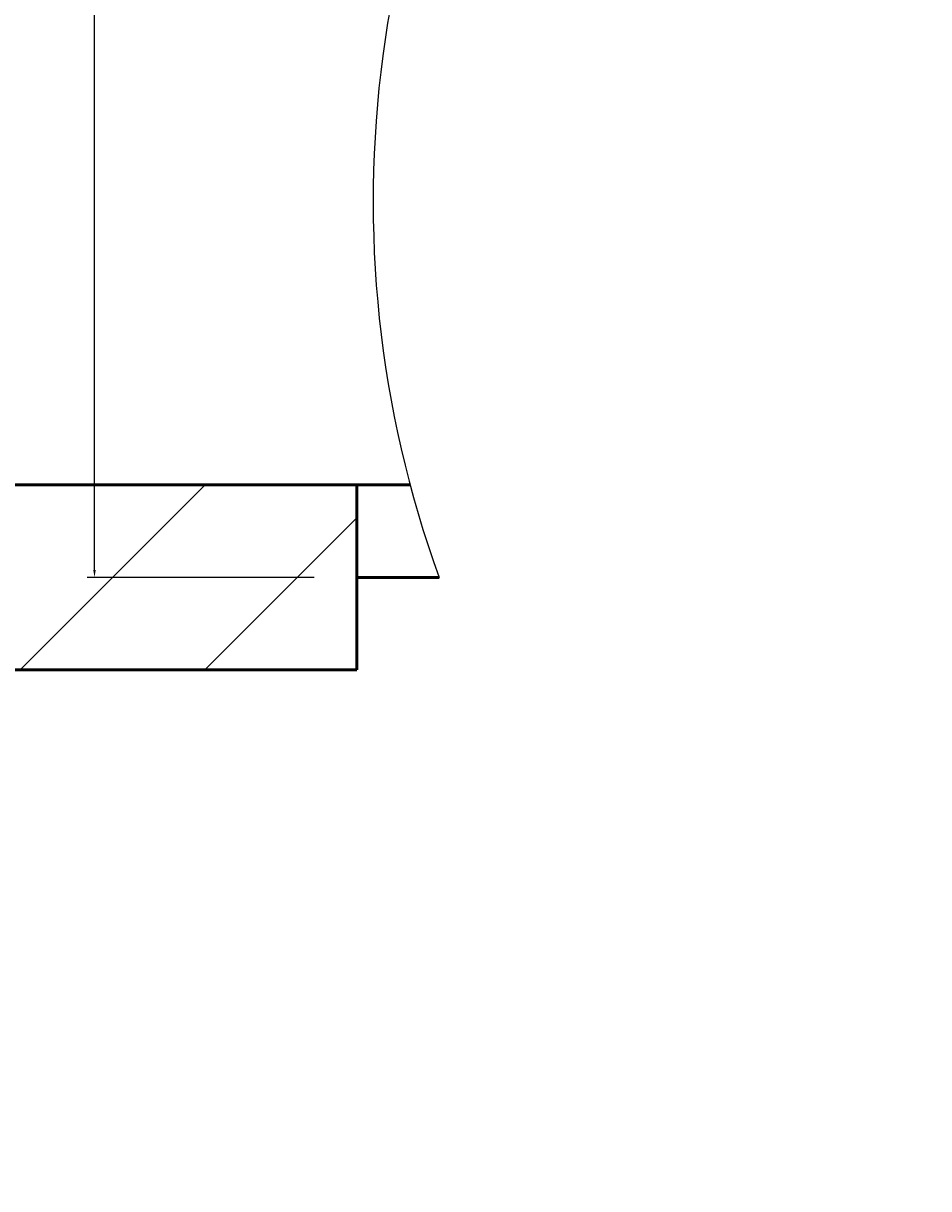
# Model space of a CAD drawing. Units: inches. Extents: x 1901 to 2863, y 888 to 2433.
# Tile 74 of 91: x 2564 to 2586, y 2066 to 2094. Entities that reach past the tile are written whole.
import ezdxf

# ---------------------------------------------------------------- set-up
doc = ezdxf.new("R2010")
doc.units = ezdxf.units.IN
for name, color, linetype, lineweight in [('A-ANNO-DIMS', 2, 'Continuous', 18), ('A-DOOR', 4, 'Continuous', 25), ('A-WALL', 7, 'Continuous', 50), ('A-WALL-PATT', 8, 'Continuous', 13)]:
    doc.layers.add(name, color=color, linetype=linetype, lineweight=lineweight)
doc.styles.get("Standard").update_dxf_attribs({"font": 'arial.ttf'})
doc.dimstyles.get("Standard").update_dxf_attribs({"dimtxt": 0.18, "dimasz": 0.18, "dimexe": 0.18, "dimexo": 0.0625, "dimgap": 0.09, "dimtad": 0, "dimtih": 1, "dimtoh": 1, "dimdec": 4, "dimzin": 0, "dimdsep": 46, "dimtxsty": 'Standard', "dimcen": 0.09, "dimadec": 0, "dimazin": 0, "dimtfac": 1, "dimtdec": 4, "dimtofl": 0, "dimtmove": 0, "dimatfit": 3, "dimfxl": 1, "dimtolj": 1, "dimtzin": 0, "dimarcsym": 0})

# ---------------------------------------------------------------- blocks, each defined once
blk = doc.blocks.new('DOOR-27')
blk.add_arc((26.814, 9.122), 26.862, 90, 199.8893)
blk = doc.blocks.new('*D35')
at = {"layer": 'A-ANNO-DIMS', "color": 0, "lineweight": -2, "transparency": 16777216}
for p, q in [((2570.714, 2116.884), (2565.196, 2116.884)), ((2565.376, 2116.704), (2565.376, 2099.067)), ((2565.376, 2081.064), (2565.376, 2098.701)), ((2570.714, 2080.884), (2565.196, 2080.884))]:
    blk.add_line(p, q, dxfattribs=at)
at = {"layer": 'A-ANNO-DIMS', "color": 0, "transparency": 16777216}
for points in [[(2565.346, 2116.704), (2565.406, 2116.704), (2565.376, 2116.884)], [(2565.346, 2081.064), (2565.406, 2081.064), (2565.376, 2080.884)]]:
    blk.add_solid(points, dxfattribs=at)
at = {"layer": 'Defpoints', "color": 0, "transparency": 16777216}
for p in [(2565.376, 2116.884), (2570.776, 2116.884), (2570.776, 2080.884)]:
    blk.add_point(p, dxfattribs=at)
at = {"layer": 'A-ANNO-DIMS', "color": 0, "transparency": 16777216, "insert": (2565.376, 2098.884), "char_height": 0.18, "attachment_point": 5}
blk.add_mtext('\\A1;DOOR D3 36 TYP.', dxfattribs=at)

msp = doc.modelspace()

# ---------------------------------------------------------------- hatches: boundary and pattern name
at = {"layer": 'A-WALL-PATT'}
h = msp.add_hatch(dxfattribs=at)
h.set_pattern_fill('ANSI32', color=256)
h.paths.add_polyline_path([(2443.926, 2139.888), (2439.426, 2139.888), (2439.426, 2069.348), (2441.676, 2069.348), (2443.926, 2069.348), (2443.926, 2078.634), (2521.926, 2078.634), (2521.926, 2075.067), (2524.176, 2075.067), (2526.426, 2075.067), (2526.426, 2078.634), (2571.755, 2078.634), (2571.755, 2080.884), (2571.755, 2083.134), (2443.926, 2083.134)])
h.paths.add_polyline_path([(2526.426, 2054.634), (2524.176, 2054.634), (2521.926, 2054.634), (2521.926, 2030.634), (2443.926, 2030.634), (2443.926, 2045.348), (2439.426, 2045.348), (2439.426, 1983.867), (2443.926, 1983.867), (2443.926, 2026.134), (2521.926, 2026.134), (2526.426, 2026.134)])
h.paths.add_polyline_path([(2443.926, 1923.867), (2439.426, 1923.867), (2439.426, 1872.634), (2443.926, 1872.634)])
h.paths.add_polyline_path([(2636.233, 1766.134), (2609.926, 1766.134), (2609.926, 1779.785), (2605.426, 1779.785), (2605.426, 1766.134), (2486.614, 1766.134), (2486.614, 1770.671), (2482.114, 1770.671), (2482.114, 1766.134), (2482.114, 1761.634), (2636.233, 1761.634), (2636.233, 1763.884)])
h.paths.add_polyline_path([(2519.536, 1663.384), (2519.536, 1665.634), (2494.926, 1665.634), (2481.831, 1665.634), (2481.831, 1663.384), (2481.831, 1661.134), (2490.426, 1661.134), (2490.426, 1640.157), (2494.926, 1640.157), (2494.926, 1661.134), (2519.536, 1661.134)])
h.paths.add_polyline_path([(2443.926, 1712.134), (2443.926, 1716.634), (2414.464, 1716.634), (2414.464, 1712.134), (2439.426, 1712.134), (2439.426, 1545.507), (2443.926, 1545.507), (2443.926, 1661.134), (2448.475, 1661.134), (2448.475, 1665.634), (2443.926, 1665.634)])
h.paths.add_polyline_path([(2343.426, 1712.134), (2365.525, 1712.134), (2365.525, 1714.384), (2365.525, 1716.634), (2333.871, 1716.634), (2333.871, 1714.384), (2333.871, 1712.134), (2338.926, 1712.134), (2338.926, 1575.634), (2338.926, 1545.507), (2343.426, 1545.507), (2343.426, 1547.507), (2343.426, 1580.134)])
h.paths.add_polyline_path([(2752.926, 1665.634), (2579.536, 1665.634), (2579.536, 1661.134), (2615.926, 1661.134), (2615.926, 1529.134), (2598.931, 1529.134), (2598.931, 1524.634), (2623.127, 1524.634), (2623.127, 1526.884), (2623.127, 1529.134), (2620.426, 1529.134), (2620.426, 1661.134), (2748.426, 1661.134), (2748.426, 1633.499), (2752.926, 1633.499)])
h.paths.add_polyline_path([(2752.926, 1419.929), (2748.426, 1419.929), (2748.426, 1400.134), (2659.426, 1400.134), (2659.426, 1444.333), (2657.176, 1444.333), (2654.926, 1444.333), (2654.926, 1400.134), (2643.649, 1400.134), (2643.649, 1395.634), (2748.426, 1395.634), (2748.426, 1364.035), (2752.926, 1364.035)])
h.paths.add_polyline_path([(2752.926, 1492.878), (2748.426, 1492.878), (2748.426, 1476.634), (2667.426, 1476.634), (2667.426, 1479.71), (2665.176, 1479.71), (2662.926, 1479.71), (2662.926, 1476.634), (2654.926, 1476.634), (2654.926, 1469.536), (2659.426, 1469.536), (2659.426, 1472.134), (2748.426, 1472.134), (2748.426, 1455.929), (2752.926, 1455.929)])
h.paths.add_polyline_path([(2752.926, 1304.035), (2748.426, 1304.035), (2748.426, 1263.634), (2738.66, 1263.634), (2738.66, 1259.134), (2752.926, 1259.134)])
h.paths.add_polyline_path([(2685.926, 1259.134), (2695.49, 1259.134), (2695.49, 1261.384), (2695.49, 1263.634), (2677.837, 1263.634), (2677.837, 1261.384), (2677.837, 1259.134), (2681.426, 1259.134), (2681.426, 1203.634), (2653.277, 1203.634), (2653.277, 1199.134), (2685.926, 1199.134), (2685.926, 1203.634)])
h.paths.add_polyline_path([(2609.426, 1395.634), (2611.848, 1395.634), (2611.848, 1400.134), (2598.888, 1400.134), (2598.888, 1397.884), (2598.888, 1395.634), (2604.926, 1395.634), (2604.926, 1268.134), (2554.726, 1268.134), (2554.726, 1265.884), (2554.726, 1263.634), (2604.926, 1263.634), (2604.926, 1203.634), (2571.306, 1203.634), (2571.306, 1199.134), (2604.926, 1199.134), (2629.277, 1199.134), (2629.277, 1201.384), (2629.277, 1203.634), (2609.426, 1203.634), (2609.426, 1258.634), (2609.426, 1259.134), (2654.804, 1259.134), (2654.804, 1263.634), (2609.426, 1263.634)])
h.paths.add_polyline_path([(2443.926, 1304.035), (2439.426, 1304.035), (2439.426, 1259.134), (2443.926, 1259.134), (2456.16, 1259.134), (2456.16, 1261.384), (2456.16, 1263.634), (2443.926, 1263.634)])
h.paths.add_polyline_path([(2525.426, 1263.634), (2531.778, 1263.634), (2531.778, 1268.134), (2520.926, 1268.134), (2520.926, 1263.634), (2511.409, 1263.634), (2511.409, 1259.134), (2520.926, 1259.134), (2520.926, 1199.134), (2547.306, 1199.134), (2547.306, 1201.384), (2547.306, 1203.634), (2525.426, 1203.634)])
h.paths.add_polyline_path([(2443.926, 1434.842), (2439.426, 1434.842), (2439.426, 1364.035), (2441.676, 1364.035), (2443.926, 1364.035)])
h.paths.add_polyline_path([(2567.134, 1400.134), (2443.926, 1400.134), (2443.926, 1395.634), (2567.134, 1395.634)])
h.paths.add_polyline_path([(2443.926, 1545.507), (2439.426, 1545.507), (2439.426, 1494.842), (2443.926, 1494.842)])
h.paths.add_polyline_path([(2494.926, 1553.349), (2492.676, 1553.349), (2490.426, 1553.349), (2490.426, 1524.634), (2494.926, 1524.634), (2525.936, 1524.634), (2525.936, 1526.884), (2525.936, 1529.134), (2494.926, 1529.134)])
h.paths.add_polyline_path([(2752.926, 1573.499), (2748.426, 1573.499), (2748.426, 1529.134), (2657.759, 1529.134), (2657.759, 1524.634), (2662.926, 1524.634), (2662.926, 1498.631), (2667.426, 1498.631), (2667.426, 1524.634), (2748.426, 1524.634), (2748.426, 1516.878), (2752.926, 1516.878)])
h.paths.add_polyline_path([(2038.602, 2237.418), (2080.174, 2237.418), (2080.174, 2256.075), (2038.602, 2256.075)], flags=9)
h.paths.add_polyline_path([(2292.009, 1062.394), (2539.932, 1062.394), (2539.932, 1099.487), (2292.009, 1099.487)], flags=9)
h.paths.add_polyline_path([(2424.91, 1832.253), (2448.513, 1832.253), (2448.513, 1846.678), (2424.91, 1846.678)], flags=9)
h.paths.add_polyline_path([(2359.076, 1832.253), (2382.678, 1832.253), (2382.678, 1846.678), (2359.076, 1846.678)], flags=9)
h.paths.add_polyline_path([(2352.899, 1684.802), (2367.543, 1684.802), (2367.543, 1697.167), (2352.899, 1697.167)], flags=9)
h.paths.add_polyline_path([(2079.288, 1755.826), (2169.024, 1755.826), (2169.024, 1774.372), (2079.288, 1774.372)], flags=9)
h.paths.add_polyline_path([(2404.09, 1373.857), (2404.09, 1463.593), (2385.544, 1463.593), (2385.544, 1373.857)], flags=9)
h.paths.add_polyline_path([(2268.091, 2236.371), (2309.636, 2236.371), (2309.636, 2255.028), (2268.091, 2255.028)], flags=9)
h.paths.add_polyline_path([(2575.96, 1700.951), (2665.696, 1700.951), (2665.696, 1719.498), (2575.96, 1719.498)], flags=9)
h.paths.add_polyline_path([(2302.962, 1878.474), (2329.524, 1878.474), (2329.524, 1888.777), (2302.962, 1888.777)], flags=9)
h.paths.add_polyline_path([(2097.415, 2240.576), (2126.573, 2240.576), (2126.573, 2259.233), (2097.415, 2259.233)], flags=9)
h.paths.add_polyline_path([(2208.725, 2246.124), (2237.882, 2246.124), (2237.882, 2264.781), (2208.725, 2264.781)], flags=9)
h.paths.add_polyline_path([(2038.147, 1925.958), (2076.987, 1925.958), (2076.987, 1944.615), (2038.147, 1944.615)], flags=9)
h.paths.add_polyline_path([(2239.144, 1926.672), (2288.465, 1926.672), (2288.465, 1945.329), (2239.144, 1945.329)], flags=9)
h.paths.add_polyline_path([(2175.429, 2007.33), (2212.356, 2007.33), (2212.356, 2025.987), (2175.429, 2025.987)], flags=9)
h.paths.add_polyline_path([(2225.034, 2091.794), (2263.875, 2091.794), (2263.875, 2110.451), (2225.034, 2110.451)], flags=9)
h.paths.add_polyline_path([(2035.398, 2098.478), (2074.238, 2098.478), (2074.238, 2117.135), (2035.398, 2117.135)], flags=9)
h.paths.add_polyline_path([(2050.102, 2029.209), (2083.26, 2029.209), (2083.26, 2047.866), (2050.102, 2047.866)], flags=9)
h.paths.add_polyline_path([(2069.677, 1956.719), (2098.835, 1956.719), (2098.835, 1975.376), (2069.677, 1975.376)], flags=9)
h.paths.add_polyline_path([(2328.62, 1753.336), (2361.663, 1753.336), (2361.663, 1771.993), (2328.62, 1771.993)], flags=9)
h.paths.add_polyline_path([(2395.162, 2060.888), (2395.162, 2140.654), (2378.676, 2140.654), (2378.676, 2060.888)], flags=9)
h.paths.add_polyline_path([(2463.728, 2059.02), (2492.886, 2059.02), (2492.886, 2077.677), (2463.728, 2077.677)], flags=9)
h.paths.add_polyline_path([(2458.027, 2181.536), (2496.868, 2181.536), (2496.868, 2200.194), (2458.027, 2200.194)], flags=9)
h.paths.add_polyline_path([(2456.855, 2228.831), (2498.401, 2228.831), (2498.401, 2247.488), (2456.855, 2247.488)], flags=9)
h.paths.add_polyline_path([(2527.577, 2243.074), (2556.735, 2243.074), (2556.735, 2261.731), (2527.577, 2261.731)], flags=9)
h.paths.add_polyline_path([(2694.461, 2232.767), (2736.033, 2232.767), (2736.033, 2251.425), (2694.461, 2251.425)], flags=9)
h.paths.add_polyline_path([(2637.821, 2249.225), (2666.979, 2249.225), (2666.979, 2267.882), (2637.821, 2267.882)], flags=9)
h.paths.add_polyline_path([(2623.687, 2183.541), (2662.528, 2183.541), (2662.528, 2202.199), (2623.687, 2202.199)], flags=9)
h.paths.add_polyline_path([(2691.965, 2021.5), (2725.124, 2021.5), (2725.124, 2040.157), (2691.965, 2040.157)], flags=9)
h.paths.add_polyline_path([(2621.043, 1975.912), (2662.335, 1975.912), (2662.335, 1994.569), (2621.043, 1994.569)], flags=9)
h.paths.add_polyline_path([(2479.032, 1927.62), (2519.844, 1927.62), (2519.844, 1946.277), (2479.032, 1946.277)], flags=9)
h.paths.add_polyline_path([(2670.941, 1849.076), (2716.005, 1849.076), (2716.005, 1867.734), (2670.941, 1867.734)], flags=9)
h.paths.add_polyline_path([(2523.613, 1782.956), (2550.175, 1782.956), (2550.175, 1793.26), (2523.613, 1793.26)], flags=9)
h.paths.add_polyline_path([(2450.841, 1207.331), (2492.386, 1207.331), (2492.386, 1225.989), (2450.841, 1225.989)], flags=9)
h.paths.add_polyline_path([(2527.751, 1203.841), (2556.908, 1203.841), (2556.908, 1222.499), (2527.751, 1222.499)], flags=9)
h.paths.add_polyline_path([(2639.111, 1207.2), (2668.268, 1207.2), (2668.268, 1225.857), (2639.111, 1225.857)], flags=9)
h.paths.add_polyline_path([(2692.594, 1218.965), (2734.167, 1218.965), (2734.167, 1237.623), (2692.594, 1237.623)], flags=9)
h.paths.add_polyline_path([(2669.266, 1366.329), (2708.106, 1366.329), (2708.106, 1384.987), (2669.266, 1384.987)], flags=25)
h.paths.add_polyline_path([(2463.313, 1358.031), (2502.153, 1358.031), (2502.153, 1376.688), (2463.313, 1376.688)], flags=9)
h.paths.add_polyline_path([(2494.725, 1449.963), (2531.652, 1449.963), (2531.652, 1468.62), (2494.725, 1468.62)], flags=9)
h.paths.add_polyline_path([(2675.565, 1422.157), (2708.724, 1422.157), (2708.724, 1440.815), (2675.565, 1440.815)], flags=25)
h.paths.add_polyline_path([(2685.634, 1493.891), (2714.792, 1493.891), (2714.792, 1512.548), (2685.634, 1512.548)], flags=9)
h.paths.add_polyline_path([(2686.805, 1529.913), (2725.645, 1529.913), (2725.645, 1548.57), (2686.805, 1548.57)], flags=25)
h.paths.add_polyline_path([(2503.651, 1537.991), (2552.972, 1537.991), (2552.972, 1556.648), (2503.651, 1556.648)], flags=9)
h.paths.add_polyline_path([(2291.713, 1643.504), (2318.275, 1643.504), (2318.275, 1653.807), (2291.713, 1653.807)], flags=9)
h.paths.add_polyline_path([(2450.626, 1610.52), (2477.189, 1610.52), (2477.189, 1620.824), (2450.626, 1620.824)], flags=9)
h.paths.add_polyline_path([(2359.985, 1551.814), (2422.253, 1551.814), (2422.253, 1562.117), (2359.985, 1562.117)], flags=9)
h.paths.add_polyline_path([(2280.106, 1249.006), (2321.651, 1249.006), (2321.651, 1267.663), (2280.106, 1267.663)], flags=9)
h.paths.add_polyline_path([(2164.057, 1274.232), (2193.215, 1274.232), (2193.215, 1292.889), (2164.057, 1292.889)], flags=9)
h.paths.add_polyline_path([(2118.21, 1277.694), (2151.252, 1277.694), (2151.252, 1296.351), (2118.21, 1296.351)], flags=9)
h.paths.add_polyline_path([(2031.946, 1268.529), (2073.519, 1268.529), (2073.519, 1287.187), (2031.946, 1287.187)], flags=9)
h.paths.add_polyline_path([(2050.199, 1409.079), (2089.04, 1409.079), (2089.04, 1427.736), (2050.199, 1427.736)], flags=9)
h.paths.add_polyline_path([(2243.743, 1421.032), (2282.584, 1421.032), (2282.584, 1439.689), (2243.743, 1439.689)], flags=9)
h.paths.add_polyline_path([(2190.746, 1509.769), (2231.558, 1509.769), (2231.558, 1528.426), (2190.746, 1528.426)], flags=9)
h.paths.add_polyline_path([(2058.392, 1475.415), (2091.55, 1475.415), (2091.55, 1494.073), (2058.392, 1494.073)], flags=9)
h.paths.add_polyline_path([(2062.447, 1553.09), (2091.605, 1553.09), (2091.605, 1571.747), (2062.447, 1571.747)], flags=9)
h.paths.add_polyline_path([(2219.524, 1590.365), (2266.147, 1590.365), (2266.147, 1609.022), (2219.524, 1609.022)], flags=9)
h.paths.add_polyline_path([(2041.072, 1584.188), (2079.912, 1584.188), (2079.912, 1602.845), (2041.072, 1602.845)], flags=9)

# ---------------------------------------------------------------- linework, layer by layer
at = {"layer": 'A-WALL'}
for p, q in [((2443.926, 2083.134), (2573.051, 2083.134)), ((2571.755, 2083.134), (2571.755, 2078.634)), ((2571.755, 2078.634), (2571.755, 2080.884)), ((2571.755, 2080.884), (2573.755, 2080.884)), ((2526.426, 2078.634), (2571.755, 2078.634))]:
    msp.add_line(p, q, dxfattribs=at)

# ---------------------------------------------------------------- block references
at = {"layer": 'A-DOOR'}
msp.add_blockref('DOOR-27', (2572.2, 2080.9), dxfattribs=at)

# ---------------------------------------------------------------- dimensions: what is measured, and where the dimension line sits
at = {"layer": 'A-ANNO-DIMS'}
dim = msp.add_linear_dim(base=(2565.376, 2116.884), p1=(2570.776, 2080.884), p2=(2570.776, 2116.884), angle=90, text='DOOR D3 <> TYP.', dimstyle='Standard', override={"dimdec": 0, "dimlfac": 1, "dimrnd": 0, "dimzin": 0, "dimdsep": 46, "dimlunit": 2}, dxfattribs=at)
dim.commit()
dim.dimension.update_dxf_attribs({"geometry": '*D35', "text_midpoint": (2565.376, 2098.884)})

doc.saveas('drawing.dxf')
